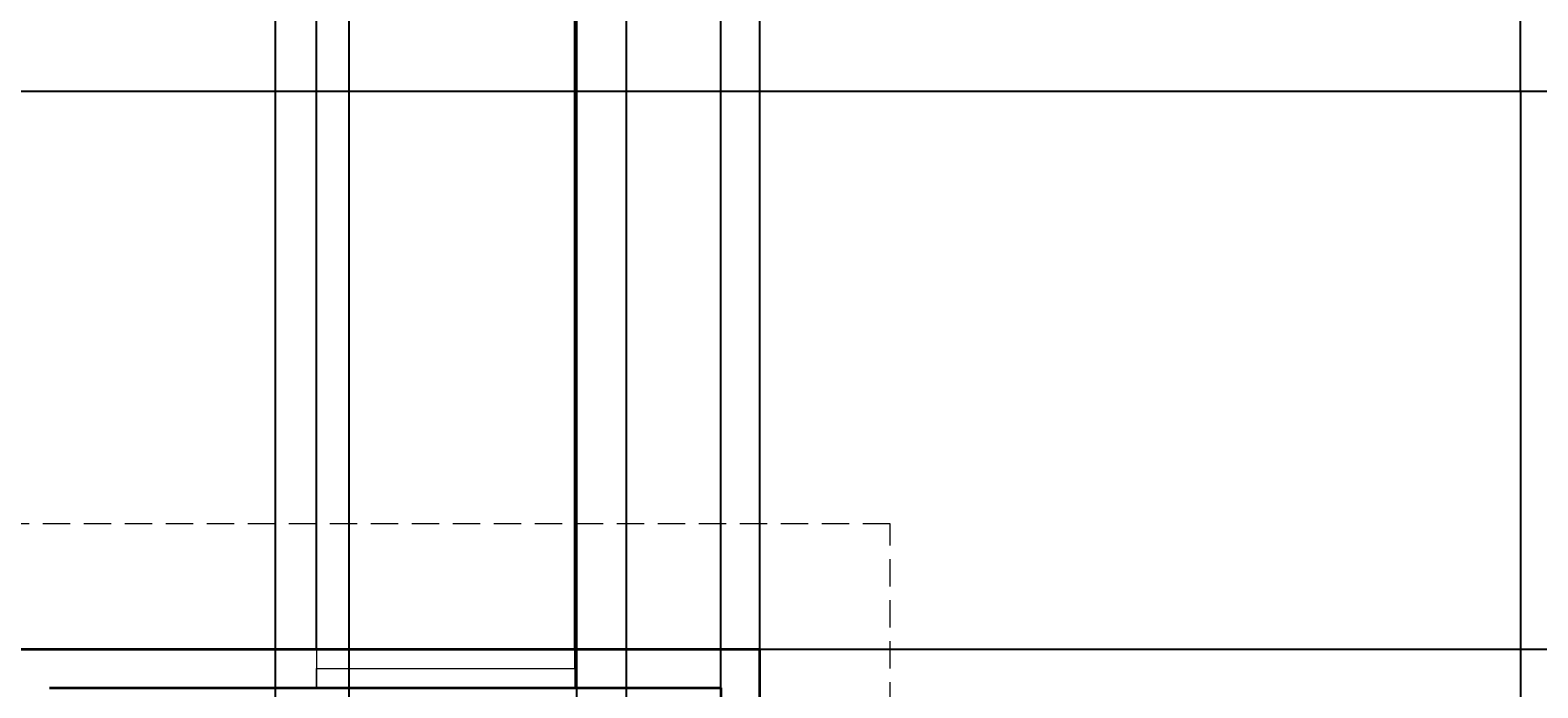
# Model space of a CAD drawing. Units: inches. Extents: x 1770 to 2988, y 1161 to 3221.
# Tile 31 of 44: x 2456 to 2807, y 2368 to 2520. Entities that reach past the tile are written whole.
import ezdxf

# ---------------------------------------------------------------- set-up
doc = ezdxf.new("R2010")
doc.units = ezdxf.units.IN
doc.linetypes.add('DASHED2', pattern=[9.525, 6.35, -3.175])
for name, color, linetype, lineweight in [('A-ANNO-DIMS', 2, 'Continuous', 18), ('A-GLAZ', 4, 'Continuous', 18), ('A-ROOF-OVHD', 7, 'DASHED2', 18), ('A-WALL', 7, 'Continuous', 35), ('C-PROP', 7, 'Continuous', 25)]:
    doc.layers.add(name, color=color, linetype=linetype, lineweight=lineweight)
doc.styles.get("Standard").update_dxf_attribs({"font": 'arial.ttf'})
doc.dimstyles.get("Standard").update_dxf_attribs({"dimtxt": 0.18, "dimasz": 0.18, "dimexe": 0.18, "dimexo": 0.0625, "dimgap": 0.09, "dimtad": 0, "dimtih": 1, "dimtoh": 1, "dimdec": 4, "dimzin": 0, "dimdsep": 46, "dimtxsty": 'Standard', "dimcen": 0.09, "dimadec": 0, "dimazin": 0, "dimtfac": 1, "dimtdec": 4, "dimtofl": 0, "dimtmove": 0, "dimatfit": 3, "dimfxl": 1, "dimtolj": 1, "dimtzin": 0, "dimarcsym": 0})

# ---------------------------------------------------------------- blocks, each defined once
blk = doc.blocks.new('WIN-60-EXT')
for p, q in [((0, 9), (0, 0)), ((60, 4.5), (60, 9)), ((60, 9), (60, 0)), ((0, 0), (0, 4.5)), ((0, 4.5), (60, 4.5))]:
    blk.add_line(p, q)
blk = doc.blocks.new('*D56')
at = {"layer": 'A-ANNO-DIMS', "color": 0, "lineweight": -2, "transparency": 16777216}
for p, q in [((1971.53, 2506.34), (1971.53, 2570.7)), ((1971.71, 2570.52), (2386.59, 2570.52)), ((2802.26, 2570.52), (2387.38, 2570.52)), ((2802.44, 2506.34), (2802.44, 2570.7))]:
    blk.add_line(p, q, dxfattribs=at)
at = {"layer": 'A-ANNO-DIMS', "color": 0, "transparency": 16777216}
for points in [[(1971.71, 2570.55), (1971.71, 2570.49), (1971.53, 2570.52)], [(2802.26, 2570.55), (2802.26, 2570.49), (2802.44, 2570.52)]]:
    blk.add_solid(points, dxfattribs=at)
at = {"layer": 'Defpoints', "color": 0, "transparency": 16777216}
for p in [(2802.44, 2570.52), (1971.53, 2506.27), (2802.44, 2506.27)]:
    blk.add_point(p, dxfattribs=at)
at = {"layer": 'A-ANNO-DIMS', "color": 0, "transparency": 16777216, "insert": (2386.99, 2570.52), "char_height": 0.18, "attachment_point": 5}
blk.add_mtext('\\A1;830.9', dxfattribs=at)
blk = doc.blocks.new('*D59')
at = {"layer": 'A-ANNO-DIMS', "color": 0, "lineweight": -2, "transparency": 16777216}
for p, q in [((2802.5, 2506.27), (2866.87, 2506.27)), ((2866.69, 2506.09), (2866.69, 2441.67)), ((2866.69, 2376.88), (2866.69, 2441.31)), ((2625.76, 2376.7), (2866.87, 2376.7))]:
    blk.add_line(p, q, dxfattribs=at)
at = {"layer": 'A-ANNO-DIMS', "color": 0, "transparency": 16777216}
for points in [[(2866.66, 2506.09), (2866.72, 2506.09), (2866.69, 2506.27)], [(2866.66, 2376.88), (2866.72, 2376.88), (2866.69, 2376.7)]]:
    blk.add_solid(points, dxfattribs=at)
at = {"layer": 'Defpoints', "color": 0, "transparency": 16777216}
for p in [(2802.44, 2506.27), (2866.69, 2506.27), (2625.7, 2376.7)]:
    blk.add_point(p, dxfattribs=at)
at = {"layer": 'A-ANNO-DIMS', "color": 0, "transparency": 16777216, "insert": (2866.69, 2441.49), "char_height": 0.18, "attachment_point": 5}
blk.add_mtext('\\A1;129.57', dxfattribs=at)
blk = doc.blocks.new('*D61')
at = {"layer": 'A-ANNO-DIMS', "color": 0, "lineweight": -2, "transparency": 16777216}
for p, q in [((2625.76, 2376.7), (2866.87, 2376.7)), ((2866.69, 2376.52), (2866.69, 1993.63)), ((2866.69, 1610.38), (2866.69, 1993.27)), ((2625.76, 1610.2), (2866.87, 1610.2))]:
    blk.add_line(p, q, dxfattribs=at)
at = {"layer": 'A-ANNO-DIMS', "color": 0, "transparency": 16777216}
for points in [[(2866.66, 2376.52), (2866.72, 2376.52), (2866.69, 2376.7)], [(2866.66, 1610.38), (2866.72, 1610.38), (2866.69, 1610.2)]]:
    blk.add_solid(points, dxfattribs=at)
at = {"layer": 'Defpoints', "color": 0, "transparency": 16777216}
for p in [(2625.7, 2376.7), (2866.69, 2376.7), (2625.7, 1610.2)]:
    blk.add_point(p, dxfattribs=at)
at = {"layer": 'A-ANNO-DIMS', "color": 0, "transparency": 16777216, "insert": (2866.69, 1993.45), "char_height": 0.18, "attachment_point": 5}
blk.add_mtext('\\A1;766.5', dxfattribs=at)
blk = doc.blocks.new('*D66')
at = {"layer": 'A-ANNO-DIMS', "color": 0, "lineweight": -2, "transparency": 16777216}
for p, q in [((2397.97, 2376.76), (2397.97, 2570.7)), ((2398.15, 2570.52), (2459.91, 2570.52)), ((2522.58, 2570.52), (2460.82, 2570.52)), ((2522.76, 2376.76), (2522.76, 2570.7))]:
    blk.add_line(p, q, dxfattribs=at)
at = {"layer": 'A-ANNO-DIMS', "color": 0, "transparency": 16777216}
for points in [[(2398.15, 2570.55), (2398.15, 2570.49), (2397.97, 2570.52)], [(2522.58, 2570.55), (2522.58, 2570.49), (2522.76, 2570.52)]]:
    blk.add_solid(points, dxfattribs=at)
at = {"layer": 'Defpoints', "color": 0, "transparency": 16777216}
for p in [(2522.76, 2570.52), (2397.97, 2376.7), (2522.76, 2376.7)]:
    blk.add_point(p, dxfattribs=at)
at = {"layer": 'A-ANNO-DIMS', "color": 0, "transparency": 16777216, "insert": (2460.36, 2570.52), "char_height": 0.18, "attachment_point": 5}
blk.add_mtext('\\A1;124.78', dxfattribs=at)
blk = doc.blocks.new('*D67')
at = {"layer": 'A-ANNO-DIMS', "color": 0, "lineweight": -2, "transparency": 16777216}
for p, q in [((2582.76, 2376.76), (2582.76, 2570.7)), ((2582.94, 2570.52), (2603.83, 2570.52)), ((2625.52, 2570.52), (2604.62, 2570.52)), ((2625.7, 2376.76), (2625.7, 2570.7))]:
    blk.add_line(p, q, dxfattribs=at)
at = {"layer": 'A-ANNO-DIMS', "color": 0, "transparency": 16777216}
for points in [[(2582.94, 2570.55), (2582.94, 2570.49), (2582.76, 2570.52)], [(2625.52, 2570.55), (2625.52, 2570.49), (2625.7, 2570.52)]]:
    blk.add_solid(points, dxfattribs=at)
at = {"layer": 'Defpoints', "color": 0, "transparency": 16777216}
for p in [(2625.7, 2570.52), (2582.76, 2376.7), (2625.7, 2376.7)]:
    blk.add_point(p, dxfattribs=at)
at = {"layer": 'A-ANNO-DIMS', "color": 0, "transparency": 16777216, "insert": (2604.23, 2570.52), "char_height": 0.18, "attachment_point": 5}
blk.add_mtext('\\A1;42.94', dxfattribs=at)
blk = doc.blocks.new('*D82')
at = {"layer": 'A-ANNO-DIMS', "color": 0, "lineweight": -2, "transparency": 16777216}
for p, q in [((2443.39, 1610.26), (2443.39, 2570.7)), ((2443.57, 2570.52), (2486.45, 2570.52)), ((2530.12, 2570.52), (2487.24, 2570.52)), ((2530.3, 1610.26), (2530.3, 2570.7))]:
    blk.add_line(p, q, dxfattribs=at)
at = {"layer": 'A-ANNO-DIMS', "color": 0, "transparency": 16777216}
for points in [[(2443.57, 2570.55), (2443.57, 2570.49), (2443.39, 2570.52)], [(2530.12, 2570.55), (2530.12, 2570.49), (2530.3, 2570.52)]]:
    blk.add_solid(points, dxfattribs=at)
at = {"layer": 'Defpoints', "color": 0, "transparency": 16777216}
for p in [(2530.3, 2570.52), (2443.39, 1610.2), (2530.3, 1610.2)]:
    blk.add_point(p, dxfattribs=at)
at = {"layer": 'A-ANNO-DIMS', "color": 0, "transparency": 16777216, "insert": (2486.85, 2570.52), "char_height": 0.18, "attachment_point": 5}
blk.add_mtext('\\A1;86.92', dxfattribs=at)
blk = doc.blocks.new('*D84')
at = {"layer": 'A-ANNO-DIMS', "color": 0, "lineweight": -2, "transparency": 16777216}
for p, q in [((2513.2, 1835.26), (2513.2, 2570.7)), ((2513.38, 2570.52), (2564.56, 2570.52)), ((2616.52, 2570.52), (2565.33, 2570.52)), ((2616.7, 1835.26), (2616.7, 2570.7))]:
    blk.add_line(p, q, dxfattribs=at)
at = {"layer": 'A-ANNO-DIMS', "color": 0, "transparency": 16777216}
for points in [[(2513.38, 2570.55), (2513.38, 2570.49), (2513.2, 2570.52)], [(2616.52, 2570.55), (2616.52, 2570.49), (2616.7, 2570.52)]]:
    blk.add_solid(points, dxfattribs=at)
at = {"layer": 'Defpoints', "color": 0, "transparency": 16777216}
for p in [(2616.7, 2570.52), (2513.2, 1835.2), (2616.7, 1835.2)]:
    blk.add_point(p, dxfattribs=at)
at = {"layer": 'A-ANNO-DIMS', "color": 0, "transparency": 16777216, "insert": (2564.95, 2570.52), "char_height": 0.18, "attachment_point": 5}
blk.add_mtext('\\A1;103.5', dxfattribs=at)
blk = doc.blocks.new('*D86')
at = {"layer": 'A-ANNO-DIMS', "color": 0, "lineweight": -2, "transparency": 16777216}
for p, q in [((2583.2, 1775.21), (2583.2, 2570.7)), ((2583.38, 2570.52), (2599.62, 2570.52)), ((2616.52, 2570.52), (2600.27, 2570.52)), ((2616.7, 1775.26), (2616.7, 2570.7))]:
    blk.add_line(p, q, dxfattribs=at)
at = {"layer": 'A-ANNO-DIMS', "color": 0, "transparency": 16777216}
for points in [[(2583.38, 2570.55), (2583.38, 2570.49), (2583.2, 2570.52)], [(2616.52, 2570.55), (2616.52, 2570.49), (2616.7, 2570.52)]]:
    blk.add_solid(points, dxfattribs=at)
at = {"layer": 'Defpoints', "color": 0, "transparency": 16777216}
for p in [(2616.7, 2570.52), (2583.2, 1775.15), (2616.7, 1775.2)]:
    blk.add_point(p, dxfattribs=at)
at = {"layer": 'A-ANNO-DIMS', "color": 0, "transparency": 16777216, "insert": (2599.95, 2570.52), "char_height": 0.18, "attachment_point": 5}
blk.add_mtext('\\A1;33.5', dxfattribs=at)
blk = doc.blocks.new('*D87')
at = {"layer": 'A-ANNO-DIMS', "color": 0, "lineweight": -2, "transparency": 16777216}
for p, q in [((2594.75, 1861.4), (2594.75, 2570.7)), ((2594.93, 2570.52), (2605.33, 2570.52)), ((2616.52, 2570.52), (2606.12, 2570.52)), ((2616.7, 1839.76), (2616.7, 2570.7))]:
    blk.add_line(p, q, dxfattribs=at)
at = {"layer": 'A-ANNO-DIMS', "color": 0, "transparency": 16777216}
for points in [[(2594.93, 2570.55), (2594.93, 2570.49), (2594.75, 2570.52)], [(2616.52, 2570.55), (2616.52, 2570.49), (2616.7, 2570.52)]]:
    blk.add_solid(points, dxfattribs=at)
at = {"layer": 'Defpoints', "color": 0, "transparency": 16777216}
for p in [(2616.7, 2570.52), (2594.75, 1861.34), (2616.7, 1839.7)]:
    blk.add_point(p, dxfattribs=at)
at = {"layer": 'A-ANNO-DIMS', "color": 0, "transparency": 16777216, "insert": (2605.72, 2570.52), "char_height": 0.18, "attachment_point": 5}
blk.add_mtext('\\A1;21.95', dxfattribs=at)

msp = doc.modelspace()

# ---------------------------------------------------------------- linework, layer by layer
at = {"layer": 'A-ROOF-OVHD'}
for p, q in [((2656.0216, 2405.7876), (2096.7313, 2405.7876)), ((2656.0216, 1610.2021), (2656.0216, 2405.7876))]:
    msp.add_line(p, q, dxfattribs=at)
at = {"layer": 'A-WALL'}
for p, q in [((2151.696, 2376.7021), (2625.696, 2376.7021)), ((2625.696, 2376.7021), (2625.696, 1610.2021)), ((2460.696, 2367.7021), (2616.696, 2367.7021)), ((2616.696, 2367.7021), (2616.696, 2175.7021))]:
    msp.add_line(p, q, dxfattribs=at)
at = {"layer": 'C-PROP'}
msp.add_lwpolyline([(1971.5344, 2506.2747), (2802.4374, 2506.2747), (2802.4374, 1323.5288), (1971.5344, 1323.5288)], close=True, dxfattribs=at)

# ---------------------------------------------------------------- block references
at = {"layer": 'A-GLAZ'}
msp.add_blockref('WIN-60-EXT', (2522.7555, 2367.702), dxfattribs=at)

# ---------------------------------------------------------------- dimensions: what is measured, and where the dimension line sits
at = {"layer": 'A-ANNO-DIMS'}
for base, p1, p2, override, picture, middle in [((2802.4374, 2570.5247), (1971.5344, 2506.2747), (2802.4374, 2506.2747), {"dimdec": 1, "dimlfac": 1, "dimrnd": 0, "dimzin": 0, "dimdsep": 46, "dimlunit": 2}, '*D56', (2386.9859, 2570.5247)), ((2522.7552, 2570.5247), (2397.9714, 2376.7021), (2522.7552, 2376.7021), {"dimdec": 2, "dimlfac": 1, "dimrnd": 0, "dimzin": 0, "dimdsep": 46, "dimlunit": 2}, '*D66', (2460.3633, 2570.5247)), ((2530.3038, 2570.5247), (2443.3863, 1610.2021), (2530.3038, 1610.2021), {"dimdec": 2, "dimlfac": 1, "dimrnd": 0, "dimzin": 0, "dimdsep": 46, "dimlunit": 2}, '*D82', (2486.8451, 2570.5247)), ((2616.696, 2570.5247), (2513.196, 1835.2021), (2616.696, 1835.2021), {"dimdec": 1, "dimlfac": 1, "dimrnd": 0, "dimzin": 0, "dimdsep": 46, "dimlunit": 2}, '*D84', (2564.946, 2570.5247)), ((2625.696, 2570.5247), (2582.7552, 2376.7021), (2625.696, 2376.7021), {"dimdec": 2, "dimlfac": 1, "dimrnd": 0, "dimzin": 0, "dimdsep": 46, "dimlunit": 2}, '*D67', (2604.2256, 2570.5247)), ((2616.696, 2570.5247), (2583.196, 1775.149), (2616.696, 1775.2021), {"dimdec": 1, "dimlfac": 1, "dimrnd": 0, "dimzin": 0, "dimdsep": 46, "dimlunit": 2}, '*D86', (2599.946, 2570.5247)), ((2616.696, 2570.5247), (2594.7479, 1861.3395), (2616.696, 1839.7021), {"dimdec": 2, "dimlfac": 1, "dimrnd": 0, "dimzin": 0, "dimdsep": 46, "dimlunit": 2}, '*D87', (2605.7219, 2570.5247))]:
    dim = msp.add_linear_dim(base=base, p1=p1, p2=p2, dimstyle='Standard', override=override, dxfattribs=at)
    dim.commit()
    dim.dimension.update_dxf_attribs({"geometry": picture, "text_midpoint": middle})
for base, p1, p2, override, picture, middle in [((2866.6874, 2506.2747), (2625.696, 2376.7021), (2802.4374, 2506.2747), {"dimdec": 2, "dimlfac": 1, "dimrnd": 0, "dimzin": 0, "dimdsep": 46, "dimlunit": 2}, '*D59', (2866.6874, 2441.4884)), ((2866.6874, 2376.7021), (2625.696, 1610.2021), (2625.696, 2376.7021), {"dimdec": 1, "dimlfac": 1, "dimrnd": 0, "dimzin": 0, "dimdsep": 46, "dimlunit": 2}, '*D61', (2866.6874, 1993.4521))]:
    dim = msp.add_linear_dim(base=base, p1=p1, p2=p2, angle=90, dimstyle='Standard', override=override, dxfattribs=at)
    dim.commit()
    dim.dimension.update_dxf_attribs({"geometry": picture, "text_midpoint": middle})

doc.saveas('drawing.dxf')
